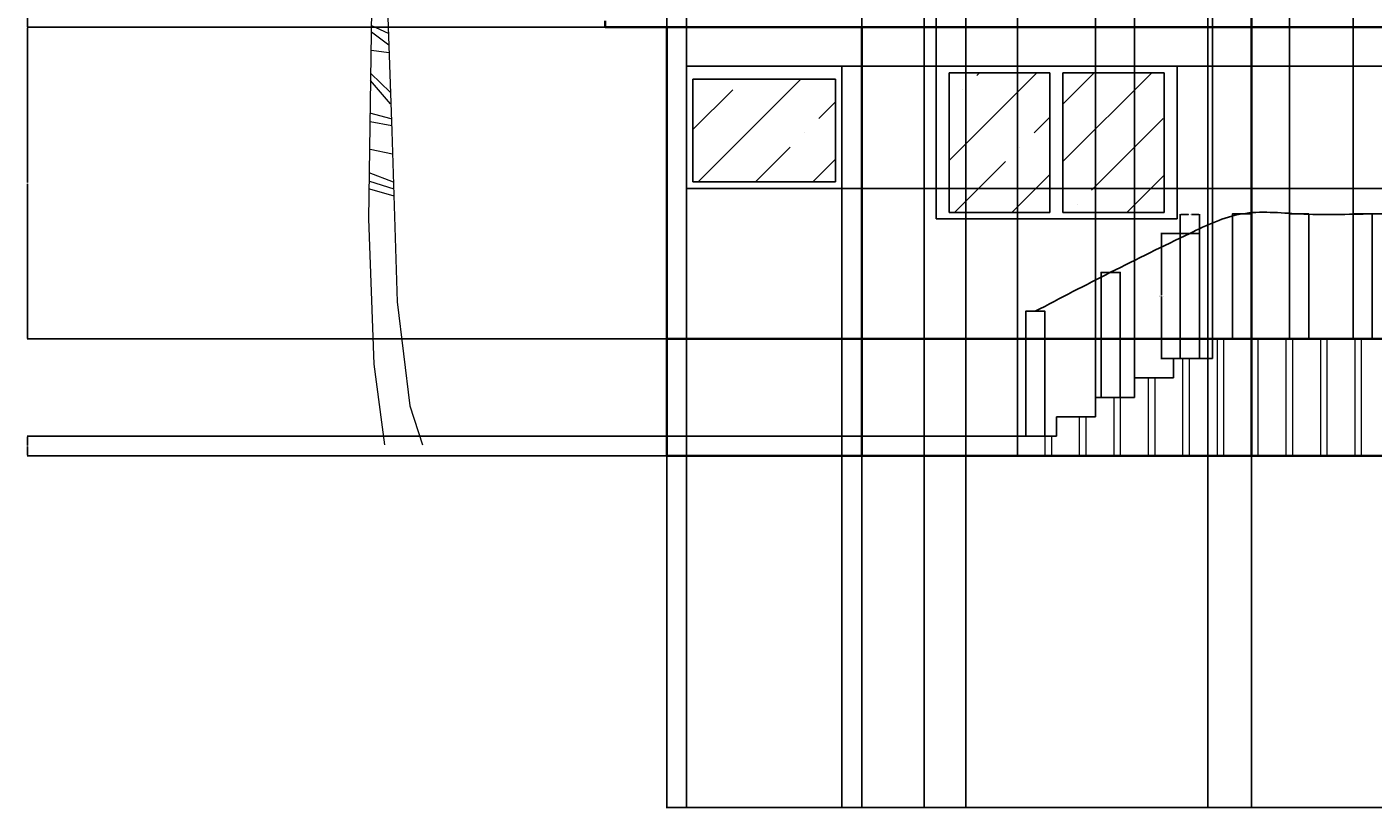
# Model space of a CAD drawing. Units: inches. Extents: x -177 to 697, y -125 to 346.
# Tile 1 of 4: x -177 to 237, y -125 to 116. Entities that reach past the tile are written whole.
import ezdxf

# ---------------------------------------------------------------- set-up
doc = ezdxf.new("R2010")
doc.units = ezdxf.units.IN
doc.header["$MEASUREMENT"] = 0
for name, color, linetype, lineweight in [('A-ANNO-DIMS', 2, 'Continuous', 18), ('A-FLOR-DECK', 8, 'Continuous', 18), ('A-FLOR-HRAL', 2, 'Continuous', 25), ('A-FLOR-STRS', 7, 'Continuous', 25), ('A-GLAZ', 4, 'Continuous', 25), ('A-GLAZ-PATT', 252, 'Continuous', 13), ('A-ROOF', 1, 'Continuous', 35), ('A-WALL', 7, 'Continuous', 35), ('L-PLNT', 94, 'Continuous', 13), ('S-FNDN', 7, 'Continuous', 35)]:
    doc.layers.add(name, color=color, linetype=linetype, lineweight=lineweight)
doc.styles.get("Standard").update_dxf_attribs({"font": 'arial.ttf'})
doc.dimstyles.get("Standard").update_dxf_attribs({"dimtxt": 0.18, "dimasz": 0.18, "dimexe": 0.18, "dimexo": 0.0625, "dimgap": 0.09, "dimtad": 0, "dimtih": 1, "dimtoh": 1, "dimdec": 4, "dimzin": 0, "dimdsep": 46, "dimtxsty": 'Standard', "dimcen": 0.09, "dimadec": 0, "dimazin": 0, "dimtfac": 1, "dimtdec": 4, "dimtofl": 0, "dimtmove": 0, "dimatfit": 3, "dimfxl": 1, "dimtolj": 1, "dimtzin": 0, "dimarcsym": 0})

# ---------------------------------------------------------------- blocks, each defined once
blk = doc.blocks.new('*U2')
for p, q in [((-7.5, 199.68), (-7.5, 197.946)), ((-5.567, 196.707), (-4.987, 201.167)), ((-4.407, 195.716), (-3.247, 200.672)), ((-2.474, 193.733), (-1.315, 199.433)), ((-6.727, 197.202), (-11.366, 197.45)), ((-3.441, 194.477), (-10.013, 195.716)), ((-1.121, 190.759), (0.232, 196.955)), ((9.317, 191.255), (10.283, 196.955)), ((11.829, 192.99), (13.182, 197.45)), ((13.956, 194.229), (14.729, 196.955)), ((15.116, 194.477), (17.822, 198.689)), ((16.082, 194.972), (17.822, 192.494)), ((18.015, 195.716), (20.914, 198.689)), ((18.015, 195.468), (18.981, 192.494)), ((19.368, 196.459), (19.948, 193.733)), ((20.914, 196.459), (21.301, 194.972)), ((21.301, 196.459), (22.847, 198.441)), ((22.074, 196.707), (23.427, 195.716)), ((23.234, 196.707), (23.62, 197.698)), ((-29.729, 190.759), (-31.469, 191.255)), ((-25.283, 191.751), (-29.342, 192.246)), ((-28.763, 190.759), (-28.763, 188.281)), ((-26.443, 191.503), (-26.636, 186.051)), ((-20.064, 191.751), (-25.863, 193.238)), ((-23.737, 191.751), (-24.51, 185.06)), ((-21.031, 191.998), (-21.804, 183.325)), ((-15.232, 191.255), (-20.644, 193.981)), ((-17.551, 191.503), (-20.451, 181.343)), ((-14.265, 190.759), (-18.131, 182.086)), ((-9.433, 189.025), (-15.618, 193.238)), ((-1.894, 192.494), (-9.24, 193.733)), ((-0.541, 189.52), (-7.307, 192.494)), ((0.038, 188.281), (1.778, 193.981)), ((1.005, 185.803), (2.358, 190.759)), ((5.837, 187.786), (7.577, 194.229)), ((11.25, 192.494), (15.889, 190.512)), ((14.536, 193.981), (17.242, 191.255)), ((-30.309, 190.512), (-30.695, 189.025)), ((-11.753, 189.768), (-15.425, 182.83)), ((-8.08, 188.034), (-12.912, 182.83)), ((-6.147, 186.299), (-9.24, 190.264)), ((-5.76, 190.016), (0.618, 185.308)), ((-5.76, 188.034), (-1.508, 182.582)), ((1.005, 182.582), (2.938, 186.547)), ((4.098, 185.06), (4.678, 190.512)), ((4.871, 186.051), (10.09, 186.547)), ((6.997, 188.529), (12.216, 187.786)), ((8.544, 190.512), (13.763, 189.52)), ((9.51, 184.317), (15.502, 188.034)), ((15.695, 186.299), (19.368, 188.777)), ((17.242, 186.547), (23.041, 180.599)), ((19.368, 187.29), (26.133, 189.768)), ((20.721, 187.042), (25.167, 181.343)), ((23.814, 187.29), (26.907, 181.343)), ((24.78, 187.538), (31.546, 188.777)), ((26.133, 187.29), (29.419, 181.838)), ((28.066, 187.29), (30.966, 182.582)), ((29.806, 186.795), (32.319, 183.078)), ((29.999, 186.795), (33.092, 187.29)), ((-4.987, 185.803), (-10.979, 182.086)), ((-3.247, 183.821), (-8.08, 181.838)), ((-2.668, 185.803), (1.198, 181.343)), ((2.938, 182.582), (6.61, 183.821)), ((4.871, 181.591), (8.544, 184.812)), ((7.77, 183.325), (16.082, 179.856)), ((11.25, 184.812), (17.628, 180.352)), ((14.536, 185.803), (19.948, 180.847)), ((32.512, 186.299), (35.218, 186.299)), ((33.479, 186.051), (34.445, 182.83)), ((35.605, 185.556), (37.151, 185.308)), ((35.798, 185.308), (36.958, 181.591)), ((38.118, 184.317), (38.504, 181.838)), ((39.857, 182.83), (40.244, 181.591)), ((-15.618, 179.36), (-20.644, 178.617)), ((-17.358, 178.617), (-13.299, 173.661)), ((-15.038, 179.36), (-10.786, 174.404)), ((-12.332, 180.104), (-9.433, 175.643)), ((-10.206, 180.104), (-8.08, 175.891)), ((-8.273, 180.104), (-6.147, 176.635)), ((-6.34, 179.608), (-4.6, 177.13)), ((-1.315, 181.591), (-5.374, 181.095)), ((-4.021, 179.36), (-2.861, 177.378)), ((-0.348, 180.352), (-1.894, 180.104)), ((4.098, 180.847), (8.35, 179.608)), ((5.644, 181.838), (13.569, 178.865)), ((7.384, 178.369), (10.476, 179.36)), ((11.829, 177.874), (18.015, 179.113)), ((18.015, 177.13), (26.133, 179.113)), ((-25.09, 175.148), (-28.376, 174.404)), ((-25.476, 174.652), (-21.224, 167.466)), ((-21.031, 177.626), (-24.897, 176.387)), ((-24.317, 175.891), (-18.711, 168.457)), ((-22.191, 176.635), (-16.391, 169.448)), ((-20.064, 177.626), (-15.812, 172.67)), ((-4.214, 175.148), (-14.072, 170.935)), ((-1.701, 176.882), (-8.66, 175.396)), ((-4.6, 174.9), (-4.021, 166.722)), ((-2.668, 176.387), (-2.376, 170.594)), ((-0.928, 176.882), (-1.508, 173.909)), ((2.551, 175.891), (-0.928, 171.431)), ((3.711, 174.404), (-0.541, 167.961)), ((1.585, 177.13), (0.038, 174.652)), ((1.585, 177.13), (6.61, 176.139)), ((2.938, 175.891), (8.737, 173.413)), ((6.224, 178.121), (8.157, 175.148)), ((8.157, 178.121), (10.476, 172.422)), ((10.476, 177.874), (12.796, 169.696)), ((13.182, 177.874), (14.729, 166.97)), ((15.889, 177.13), (16.855, 164.492)), ((18.981, 175.891), (19.561, 163.005)), ((20.914, 175.891), (30.966, 176.635)), ((21.688, 175.396), (22.074, 161.518)), ((23.814, 174.404), (25.554, 160.279)), ((-28.956, 172.174), (-32.435, 170.192)), ((-31.082, 169.944), (-32.435, 169.2)), ((-27.409, 173.413), (-30.695, 172.67)), ((-29.922, 170.687), (-27.989, 165.235)), ((-27.989, 172.422), (-26.056, 166.227)), ((-26.829, 173.661), (-23.544, 167.218)), ((-8.466, 171.678), (-16.585, 167.713)), ((-8.853, 170.935), (-7.113, 160.527)), ((-6.92, 172.917), (-5.374, 163.253)), ((5.257, 171.926), (-0.155, 163.005)), ((4.291, 173.909), (12.216, 168.953)), ((6.417, 170.439), (14.729, 164.492)), ((25.554, 173.661), (33.285, 173.661)), ((26.52, 173.165), (28.066, 159.784)), ((28.839, 172.174), (36.378, 170.687)), ((29.226, 171.926), (30.966, 158.545)), ((30.966, 170.687), (38.891, 167.713)), ((-32.628, 167.961), (-33.208, 167.961)), ((-32.628, 167.713), (-32.435, 165.979)), ((-31.662, 168.705), (-31.082, 165.483)), ((-12.139, 167.961), (-19.098, 162.014)), ((-12.719, 166.722), (-9.046, 154.828)), ((-10.979, 168.457), (-7.887, 157.801)), ((7.384, 168.705), (0.812, 157.553)), ((8.544, 165.979), (16.662, 160.527)), ((32.126, 169.696), (32.512, 158.545)), ((34.058, 168.705), (34.445, 158.545)), ((35.412, 167.713), (41.404, 164.988)), ((36.378, 166.474), (35.605, 158.792)), ((-14.265, 164.244), (-19.678, 158.049)), ((-14.265, 163.749), (-10.786, 154.828)), ((9.317, 164.244), (2.358, 154.332)), ((10.09, 162.51), (17.435, 157.058)), ((37.731, 165.235), (36.958, 159.288)), ((37.924, 165.235), (41.404, 163.749)), ((38.504, 164.492), (38.504, 159.536)), ((39.664, 163.253), (42.37, 161.766)), ((39.857, 162.757), (39.857, 160.031)), ((40.824, 161.766), (41.21, 160.031)), ((-16.005, 160.031), (-19.484, 154.084)), ((-16.585, 158.545), (-13.106, 152.35)), ((-15.618, 160.775), (-12.332, 154.332)), ((10.863, 159.784), (4.484, 152.35)), ((11.443, 157.553), (16.855, 154.332)), ((41.21, 161.518), (42.757, 160.279)), ((-18.131, 153.589), (-19.484, 151.606)), ((-17.358, 155.819), (-14.845, 151.358)), ((11.829, 155.075), (6.804, 150.119)), ((-17.938, 152.597), (-16.972, 151.111)), ((12.603, 151.111), (8.544, 148.385)), ((12.216, 153.093), (16.082, 151.606)), ((12.603, 149.872), (15.116, 149.128)), ((12.216, 148.137), (10.09, 147.393)), ((12.409, 145.659), (11.056, 145.659)), ((12.409, 146.898), (13.763, 146.402)), ((-4.081, 140.645), (0.753, 138.261)), ((-4.081, 137.547), (0.753, 135.163)), ((-4.081, 129.205), (1.124, 126.821)), ((-4.081, 127.298), (1.31, 123.246)), ((-4.081, 121.578), (1.31, 120.863)), ((-4.453, 112.283), (1.682, 105.133)), ((-4.267, 114.428), (1.682, 108.708)), ((-4.639, 102.273), (1.868, 100.604)), ((-4.453, 99.651), (2.24, 98.459)), ((-4.453, 91.071), (2.426, 89.641)), ((-4.825, 83.921), (2.612, 81.061)), ((-4.639, 81.299), (2.797, 78.916)), ((-4.639, 78.916), (2.797, 76.771))]:
    blk.add_line(p, q)
for points in [[(-2.363, 170.553), (-3.88, 148.505), (-4.988, 69.634), (-3.325, 24.869), (0, 0)], [(-0.116, 162.848), (0.554, 143.532), (2.217, 96.635), (3.88, 44.054), (7.76, 12.079), (11.64, 0)]]:
    blk.add_lwpolyline(points)
for centre, radius, start, end in [((-18.427, 181.448), 19.715, 350.285, 64.11229), ((25.595, 171.567), 25.395, 91.40319, 163.882), ((-21.738, 166.094), 25.899, 27.67115, 112.5305), ((23.687, 155.341), 32.188, 56.19272, 134.3213), ((-9.259, 151.732), 28.386, 68.38311, 147.5322), ((14.394, 148.393), 32.752, 113.7592, 177.4133), ((5.828, 132.718), 45.639, 35.98777, 95.82273), ((-32.8, 147.923), 45.309, 356.1943, 41.37848)]:
    blk.add_arc(centre, radius, start, end)
blk = doc.blocks.new('WIN-TWIN-LARGE-ELEV')
for p, q in [((0, 47.05), (74.16, 47.05)), ((0, 0), (0, 47.05)), ((74.16, 47.05), (74.16, 0)), ((4, 2), (4, 45.05)), ((4, 45.05), (35.01, 45.05)), ((35.01, 2), (35.01, 45.05)), ((39.01, 2), (39.01, 45.05)), ((39.01, 45.05), (70.16, 45.05)), ((70.16, 45.05), (70.16, 2)), ((74.16, 0), (0, 0)), ((35.01, 2), (4, 2)), ((70.16, 2), (39.01, 2))]:
    blk.add_line(p, q)
blk = doc.blocks.new('GUARD-POST-ELEV')
blk.add_lwpolyline([(5.89, 0), (0, 0), (0, 38.51), (5.89, 38.51)], close=True)
blk = doc.blocks.new('PORCH-UPRIGHT-36-ELEV')
for p, q in [((0, 36), (0, 0)), ((2, 36), (2, 0))]:
    blk.add_line(p, q)
blk = doc.blocks.new('*D15')
at = {"layer": 'A-ANNO-DIMS', "color": 0, "lineweight": -2, "transparency": 16777216}
for p, q in [((178.06, 52.19), (172.16, 52.19)), ((172.34, 52.01), (172.34, 33.12)), ((172.34, 13.86), (172.34, 32.75)), ((178.06, 13.68), (172.16, 13.68))]:
    blk.add_line(p, q, dxfattribs=at)
at = {"layer": 'A-ANNO-DIMS', "color": 0, "transparency": 16777216}
for points in [[(172.31, 52.01), (172.37, 52.01), (172.34, 52.19)], [(172.31, 13.86), (172.37, 13.86), (172.34, 13.68)]]:
    blk.add_solid(points, dxfattribs=at)
at = {"layer": 'Defpoints', "color": 0, "transparency": 16777216}
for p in [(172.34, 52.19), (178.12, 52.19), (178.12, 13.68)]:
    blk.add_point(p, dxfattribs=at)
at = {"layer": 'A-ANNO-DIMS', "color": 0, "transparency": 16777216, "insert": (172.34, 32.94), "char_height": 0.18, "attachment_point": 5}
blk.add_mtext('\\A1;POST 39 TYP.', dxfattribs=at)
blk = doc.blocks.new('*D16')
at = {"layer": 'A-ANNO-DIMS', "color": 0, "lineweight": -2, "transparency": 16777216}
for p, q in [((178.12, 52.26), (178.12, 58.15)), ((184.01, 52.26), (184.01, 58.15)), ((178.3, 57.97), (180.61, 57.97)), ((183.83, 57.97), (181.53, 57.97))]:
    blk.add_line(p, q, dxfattribs=at)
at = {"layer": 'A-ANNO-DIMS', "color": 0, "transparency": 16777216}
for points in [[(178.3, 58), (178.3, 57.94), (178.12, 57.97)], [(183.83, 58), (183.83, 57.94), (184.01, 57.97)]]:
    blk.add_solid(points, dxfattribs=at)
at = {"layer": 'Defpoints', "color": 0, "transparency": 16777216}
for p in [(184.01, 57.97), (178.12, 52.19), (184.01, 52.19)]:
    blk.add_point(p, dxfattribs=at)
at = {"layer": 'A-ANNO-DIMS', "color": 0, "transparency": 16777216, "insert": (181.07, 57.97), "char_height": 0.18, "attachment_point": 5}
blk.add_mtext('\\A1;6 TYP.', dxfattribs=at)
blk = doc.blocks.new('*D19')
at = {"layer": 'A-ANNO-DIMS', "color": 0, "lineweight": -2, "transparency": 16777216}
for p, q in [((20.05, -16.38), (20.05, -124.85)), ((500.05, -16.38), (500.05, -124.85)), ((20.23, -124.67), (259.76, -124.67)), ((499.87, -124.67), (260.34, -124.67))]:
    blk.add_line(p, q, dxfattribs=at)
at = {"layer": 'A-ANNO-DIMS', "color": 0, "transparency": 16777216}
for points in [[(20.23, -124.64), (20.23, -124.7), (20.05, -124.67)], [(499.87, -124.64), (499.87, -124.7), (500.05, -124.67)]]:
    blk.add_solid(points, dxfattribs=at)
at = {"layer": 'Defpoints', "color": 0, "transparency": 16777216}
for p in [(20.05, -16.32), (500.05, -16.32), (500.05, -124.67)]:
    blk.add_point(p, dxfattribs=at)
at = {"layer": 'A-ANNO-DIMS', "color": 0, "transparency": 16777216, "insert": (260.05, -124.67), "char_height": 0.18, "attachment_point": 5}
blk.add_mtext('\\A1;480', dxfattribs=at)
blk = doc.blocks.new('*D22')
at = {"layer": 'A-ANNO-DIMS', "color": 0, "lineweight": -2, "transparency": 16777216}
for p, q in [((79.79, 235.68), (-176.98, 235.68)), ((-176.8, 235.5), (-176.8, 175.86)), ((-176.8, 115.86), (-176.8, 175.5)), ((0.99, 115.68), (-176.98, 115.68))]:
    blk.add_line(p, q, dxfattribs=at)
at = {"layer": 'A-ANNO-DIMS', "color": 0, "transparency": 16777216}
for points in [[(-176.83, 235.5), (-176.77, 235.5), (-176.8, 235.68)], [(-176.83, 115.86), (-176.77, 115.86), (-176.8, 115.68)]]:
    blk.add_solid(points, dxfattribs=at)
at = {"layer": 'Defpoints', "color": 0, "transparency": 16777216}
for p in [(79.85, 235.68), (-176.8, 115.68), (1.05, 115.68)]:
    blk.add_point(p, dxfattribs=at)
at = {"layer": 'A-ANNO-DIMS', "color": 0, "transparency": 16777216, "insert": (-176.8, 175.68), "char_height": 0.18, "attachment_point": 5}
blk.add_mtext('\\A1;120', dxfattribs=at)
blk = doc.blocks.new('*D23')
at = {"layer": 'A-ANNO-DIMS', "color": 0, "lineweight": -2, "transparency": 16777216}
for p, q in [((19.99, 115.68), (-176.98, 115.68)), ((-176.8, 115.5), (-176.8, 67.86)), ((-176.8, 19.86), (-176.8, 67.5)), ((19.99, 19.68), (-176.98, 19.68))]:
    blk.add_line(p, q, dxfattribs=at)
at = {"layer": 'A-ANNO-DIMS', "color": 0, "transparency": 16777216}
for points in [[(-176.83, 115.5), (-176.77, 115.5), (-176.8, 115.68)], [(-176.83, 19.86), (-176.77, 19.86), (-176.8, 19.68)]]:
    blk.add_solid(points, dxfattribs=at)
at = {"layer": 'Defpoints', "color": 0, "transparency": 16777216}
for p in [(-176.8, 115.68), (20.05, 115.68), (20.05, 19.68)]:
    blk.add_point(p, dxfattribs=at)
at = {"layer": 'A-ANNO-DIMS', "color": 0, "transparency": 16777216, "insert": (-176.8, 67.68), "char_height": 0.18, "attachment_point": 5}
blk.add_mtext('\\A1;96', dxfattribs=at)
blk = doc.blocks.new('*D24')
at = {"layer": 'A-ANNO-DIMS', "color": 0, "lineweight": -2, "transparency": 16777216}
for p, q in [((128.05, -16.26), (128.05, 346.22)), ((128.23, 346.04), (157.83, 346.04)), ((187.87, 346.04), (158.27, 346.04)), ((188.05, 19.74), (188.05, 346.22))]:
    blk.add_line(p, q, dxfattribs=at)
at = {"layer": 'A-ANNO-DIMS', "color": 0, "transparency": 16777216}
for points in [[(128.23, 346.07), (128.23, 346.01), (128.05, 346.04)], [(187.87, 346.07), (187.87, 346.01), (188.05, 346.04)]]:
    blk.add_solid(points, dxfattribs=at)
at = {"layer": 'Defpoints', "color": 0, "transparency": 16777216}
for p in [(188.05, 346.04), (188.05, 19.68), (128.05, -16.32)]:
    blk.add_point(p, dxfattribs=at)
at = {"layer": 'A-ANNO-DIMS', "color": 0, "transparency": 16777216, "insert": (158.05, 346.04), "char_height": 0.18, "attachment_point": 5}
blk.add_mtext('\\A1;60', dxfattribs=at)
blk = doc.blocks.new('*D25')
at = {"layer": 'A-ANNO-DIMS', "color": 0, "lineweight": -2, "transparency": 16777216}
for p, q in [((152.05, 1.74), (152.05, 346.22)), ((152.23, 346.04), (157.84, 346.04)), ((163.87, 346.04), (158.26, 346.04)), ((164.05, 1.74), (164.05, 346.22))]:
    blk.add_line(p, q, dxfattribs=at)
at = {"layer": 'A-ANNO-DIMS', "color": 0, "transparency": 16777216}
for points in [[(152.23, 346.07), (152.23, 346.01), (152.05, 346.04)], [(163.87, 346.07), (163.87, 346.01), (164.05, 346.04)]]:
    blk.add_solid(points, dxfattribs=at)
at = {"layer": 'Defpoints', "color": 0, "transparency": 16777216}
for p in [(164.05, 346.04), (152.05, 1.68), (164.05, 1.68)]:
    blk.add_point(p, dxfattribs=at)
at = {"layer": 'A-ANNO-DIMS', "color": 0, "transparency": 16777216, "insert": (158.05, 346.04), "char_height": 0.18, "attachment_point": 5}
blk.add_mtext('\\A1;12', dxfattribs=at)
blk = doc.blocks.new('*D26')
at = {"layer": 'A-ANNO-DIMS', "color": 0, "lineweight": -2, "transparency": 16777216}
for p, q in [((127.99, -10.32), (-176.98, -10.32)), ((-176.8, -10.5), (-176.8, -13.14)), ((127.99, -16.32), (-176.98, -16.32)), ((-176.8, -16.14), (-176.8, -13.5))]:
    blk.add_line(p, q, dxfattribs=at)
at = {"layer": 'A-ANNO-DIMS', "color": 0, "transparency": 16777216}
for points in [[(-176.83, -10.5), (-176.77, -10.5), (-176.8, -10.32)], [(-176.83, -16.14), (-176.77, -16.14), (-176.8, -16.32)]]:
    blk.add_solid(points, dxfattribs=at)
at = {"layer": 'Defpoints', "color": 0, "transparency": 16777216}
for p in [(-176.8, -10.32), (128.05, -10.32), (128.05, -16.32)]:
    blk.add_point(p, dxfattribs=at)
at = {"layer": 'A-ANNO-DIMS', "color": 0, "transparency": 16777216, "insert": (-176.8, -13.32), "char_height": 0.18, "attachment_point": 5}
blk.add_mtext('\\A1;6', dxfattribs=at)
blk = doc.blocks.new('*D28')
at = {"layer": 'A-ANNO-DIMS', "color": 0, "lineweight": -2, "transparency": 16777216}
for p, q in [((211.79, 58.26), (211.79, 346.22)), ((211.97, 346.04), (221.1, 346.04)), ((231.15, 346.04), (222.01, 346.04)), ((231.33, 58.26), (231.33, 346.22))]:
    blk.add_line(p, q, dxfattribs=at)
at = {"layer": 'A-ANNO-DIMS', "color": 0, "transparency": 16777216}
for points in [[(211.97, 346.07), (211.97, 346.01), (211.79, 346.04)], [(231.15, 346.07), (231.15, 346.01), (231.33, 346.04)]]:
    blk.add_solid(points, dxfattribs=at)
at = {"layer": 'Defpoints', "color": 0, "transparency": 16777216}
for p in [(231.33, 346.04), (211.79, 58.19), (231.33, 58.19)]:
    blk.add_point(p, dxfattribs=at)
at = {"layer": 'A-ANNO-DIMS', "color": 0, "transparency": 16777216, "insert": (221.56, 346.04), "char_height": 0.18, "attachment_point": 5}
blk.add_mtext('\\A1;19.536', dxfattribs=at)
blk = doc.blocks.new('*D30')
at = {"layer": 'A-ANNO-DIMS', "color": 0, "lineweight": -2, "transparency": 16777216}
for p, q in [((20.05, 115.62), (20.05, -124.85)), ((80.05, 115.62), (80.05, -124.85)), ((20.23, -124.67), (49.83, -124.67)), ((79.87, -124.67), (50.27, -124.67))]:
    blk.add_line(p, q, dxfattribs=at)
at = {"layer": 'A-ANNO-DIMS', "color": 0, "transparency": 16777216}
for points in [[(20.23, -124.64), (20.23, -124.7), (20.05, -124.67)], [(79.87, -124.64), (79.87, -124.7), (80.05, -124.67)]]:
    blk.add_solid(points, dxfattribs=at)
at = {"layer": 'Defpoints', "color": 0, "transparency": 16777216}
for p in [(20.05, 115.68), (80.05, 115.68), (80.05, -124.67)]:
    blk.add_point(p, dxfattribs=at)
at = {"layer": 'A-ANNO-DIMS', "color": 0, "transparency": 16777216, "insert": (50.05, -124.67), "char_height": 0.18, "attachment_point": 5}
blk.add_mtext('\\A1;60', dxfattribs=at)
blk = doc.blocks.new('*D31')
at = {"layer": 'A-ANNO-DIMS', "color": 0, "lineweight": -2, "transparency": 16777216}
for p, q in [((80.05, -16.26), (80.05, 346.22)), ((80.23, 346.04), (103.83, 346.04)), ((127.87, 346.04), (104.27, 346.04)), ((128.05, -16.26), (128.05, 346.22))]:
    blk.add_line(p, q, dxfattribs=at)
at = {"layer": 'A-ANNO-DIMS', "color": 0, "transparency": 16777216}
for points in [[(80.23, 346.07), (80.23, 346.01), (80.05, 346.04)], [(127.87, 346.07), (127.87, 346.01), (128.05, 346.04)]]:
    blk.add_solid(points, dxfattribs=at)
at = {"layer": 'Defpoints', "color": 0, "transparency": 16777216}
for p in [(128.05, 346.04), (80.05, -16.32), (128.05, -16.32)]:
    blk.add_point(p, dxfattribs=at)
at = {"layer": 'A-ANNO-DIMS', "color": 0, "transparency": 16777216, "insert": (104.05, 346.04), "char_height": 0.18, "attachment_point": 5}
blk.add_mtext('\\A1;48', dxfattribs=at)
blk = doc.blocks.new('*D36')
at = {"layer": 'A-ANNO-DIMS', "color": 0, "lineweight": -2, "transparency": 16777216}
for p, q in [((26.06, 66), (26.06, -124.85)), ((73.94, 66), (73.94, -124.85)), ((26.24, -124.67), (49.6, -124.67)), ((73.76, -124.67), (50.4, -124.67))]:
    blk.add_line(p, q, dxfattribs=at)
at = {"layer": 'A-ANNO-DIMS', "color": 0, "transparency": 16777216}
for points in [[(26.24, -124.64), (26.24, -124.7), (26.06, -124.67)], [(73.76, -124.64), (73.76, -124.7), (73.94, -124.67)]]:
    blk.add_solid(points, dxfattribs=at)
at = {"layer": 'Defpoints', "color": 0, "transparency": 16777216}
for p in [(26.06, 66.06), (73.94, 66.06), (73.94, -124.67)]:
    blk.add_point(p, dxfattribs=at)
at = {"layer": 'A-ANNO-DIMS', "color": 0, "transparency": 16777216, "insert": (50, -124.67), "char_height": 0.18, "attachment_point": 5}
blk.add_mtext('\\A1;47.88', dxfattribs=at)
blk = doc.blocks.new('*D37')
at = {"layer": 'A-ANNO-DIMS', "color": 0, "lineweight": -2, "transparency": 16777216}
for p, q in [((74.01, 103.68), (697.14, 103.68)), ((696.96, 103.5), (696.96, 85.05)), ((696.96, 66.24), (696.96, 84.69)), ((74.01, 66.06), (697.14, 66.06))]:
    blk.add_line(p, q, dxfattribs=at)
at = {"layer": 'A-ANNO-DIMS', "color": 0, "transparency": 16777216}
for points in [[(696.93, 103.5), (696.99, 103.5), (696.96, 103.68)], [(696.93, 66.24), (696.99, 66.24), (696.96, 66.06)]]:
    blk.add_solid(points, dxfattribs=at)
at = {"layer": 'Defpoints', "color": 0, "transparency": 16777216}
for p in [(73.94, 103.68), (696.96, 103.68), (73.94, 66.06)]:
    blk.add_point(p, dxfattribs=at)
at = {"layer": 'A-ANNO-DIMS', "color": 0, "transparency": 16777216, "insert": (696.96, 84.87), "char_height": 0.18, "attachment_point": 5}
blk.add_mtext('\\A1;37.62', dxfattribs=at)
blk = doc.blocks.new('*D38')
at = {"layer": 'A-ANNO-DIMS', "color": 0, "lineweight": -2, "transparency": 16777216}
for p, q in [((20.05, 19.74), (20.05, 346.22)), ((20.23, 346.04), (22.75, 346.04)), ((25.88, 346.04), (23.36, 346.04)), ((26.06, 66.12), (26.06, 346.22))]:
    blk.add_line(p, q, dxfattribs=at)
at = {"layer": 'A-ANNO-DIMS', "color": 0, "transparency": 16777216}
for points in [[(20.23, 346.07), (20.23, 346.01), (20.05, 346.04)], [(25.88, 346.07), (25.88, 346.01), (26.06, 346.04)]]:
    blk.add_solid(points, dxfattribs=at)
at = {"layer": 'Defpoints', "color": 0, "transparency": 16777216}
for p in [(26.06, 346.04), (26.06, 66.06), (20.05, 19.68)]:
    blk.add_point(p, dxfattribs=at)
at = {"layer": 'A-ANNO-DIMS', "color": 0, "transparency": 16777216, "insert": (23.05, 346.04), "char_height": 0.18, "attachment_point": 5}
blk.add_mtext('\\A1;6.01', dxfattribs=at)
blk = doc.blocks.new('*D39')
at = {"layer": 'A-ANNO-DIMS', "color": 0, "lineweight": -2, "transparency": 16777216}
for p, q in [((80.05, -16.26), (80.05, 346.22)), ((80.23, 346.04), (91.11, 346.04)), ((102.79, 346.04), (91.9, 346.04)), ((102.97, 56.7), (102.97, 346.22))]:
    blk.add_line(p, q, dxfattribs=at)
at = {"layer": 'A-ANNO-DIMS', "color": 0, "transparency": 16777216}
for points in [[(80.23, 346.07), (80.23, 346.01), (80.05, 346.04)], [(102.79, 346.07), (102.79, 346.01), (102.97, 346.04)]]:
    blk.add_solid(points, dxfattribs=at)
at = {"layer": 'Defpoints', "color": 0, "transparency": 16777216}
for p in [(102.97, 346.04), (102.97, 56.63), (80.05, -16.32)]:
    blk.add_point(p, dxfattribs=at)
at = {"layer": 'A-ANNO-DIMS', "color": 0, "transparency": 16777216, "insert": (91.51, 346.04), "char_height": 0.18, "attachment_point": 5}
blk.add_mtext('\\A1;22.92', dxfattribs=at)
blk = doc.blocks.new('*D46')
at = {"layer": 'A-ANNO-DIMS', "color": 0, "lineweight": -2, "transparency": 16777216}
for p, q in [((112.1, 190.16), (112.1, -124.85)), ((186.62, 190.16), (186.62, -124.85)), ((112.28, -124.67), (148.96, -124.67)), ((186.44, -124.67), (149.75, -124.67))]:
    blk.add_line(p, q, dxfattribs=at)
at = {"layer": 'A-ANNO-DIMS', "color": 0, "transparency": 16777216}
for points in [[(112.28, -124.64), (112.28, -124.7), (112.1, -124.67)], [(186.44, -124.64), (186.44, -124.7), (186.62, -124.67)]]:
    blk.add_solid(points, dxfattribs=at)
at = {"layer": 'Defpoints', "color": 0, "transparency": 16777216}
for p in [(112.1, 190.22), (186.62, 190.22), (186.62, -124.67)]:
    blk.add_point(p, dxfattribs=at)
at = {"layer": 'A-ANNO-DIMS', "color": 0, "transparency": 16777216, "insert": (149.36, -124.67), "char_height": 0.18, "attachment_point": 5}
blk.add_mtext('\\A1;74.52', dxfattribs=at)
blk = doc.blocks.new('*D51')
at = {"layer": 'A-ANNO-DIMS', "color": 0, "lineweight": -2, "transparency": 16777216}
for p, q in [((99.22, 235.62), (99.22, -124.85)), ((200.05, 235.62), (200.05, -124.85)), ((99.4, -124.67), (149.18, -124.67)), ((199.87, -124.67), (150.09, -124.67))]:
    blk.add_line(p, q, dxfattribs=at)
at = {"layer": 'A-ANNO-DIMS', "color": 0, "transparency": 16777216}
for points in [[(99.4, -124.64), (99.4, -124.7), (99.22, -124.67)], [(199.87, -124.64), (199.87, -124.7), (200.05, -124.67)]]:
    blk.add_solid(points, dxfattribs=at)
at = {"layer": 'Defpoints', "color": 0, "transparency": 16777216}
for p in [(99.22, 235.68), (200.05, 235.68), (200.05, -124.67)]:
    blk.add_point(p, dxfattribs=at)
at = {"layer": 'A-ANNO-DIMS', "color": 0, "transparency": 16777216, "insert": (149.63, -124.67), "char_height": 0.18, "attachment_point": 5}
blk.add_mtext('\\A1;100.83', dxfattribs=at)
blk = doc.blocks.new('*D55')
at = {"layer": 'A-ANNO-DIMS', "color": 0, "lineweight": -2, "transparency": 16777216}
for p, q in [((20.05, 115.74), (20.05, 346.22)), ((20.23, 346.04), (59.24, 346.04)), ((99.04, 346.04), (60.03, 346.04)), ((99.22, 163.74), (99.22, 346.22))]:
    blk.add_line(p, q, dxfattribs=at)
at = {"layer": 'A-ANNO-DIMS', "color": 0, "transparency": 16777216}
for points in [[(20.23, 346.07), (20.23, 346.01), (20.05, 346.04)], [(99.04, 346.07), (99.04, 346.01), (99.22, 346.04)]]:
    blk.add_solid(points, dxfattribs=at)
at = {"layer": 'Defpoints', "color": 0, "transparency": 16777216}
for p in [(99.22, 346.04), (99.22, 163.68), (20.05, 115.68)]:
    blk.add_point(p, dxfattribs=at)
at = {"layer": 'A-ANNO-DIMS', "color": 0, "transparency": 16777216, "insert": (59.63, 346.04), "char_height": 0.18, "attachment_point": 5}
blk.add_mtext('\\A1;79.17', dxfattribs=at)

msp = doc.modelspace()

# ---------------------------------------------------------------- hatches: boundary and pattern name
at = {"layer": 'A-GLAZ-PATT'}
h = msp.add_hatch(dxfattribs=at)
h.set_pattern_fill('ANSI35', color=256, scale=100)
h.set_pattern_definition([(45, (-118.808, -115.734), (-17.6777, 17.6777), []), (45, (-101.13, -115.734), (-17.6777, 17.6777), [31.25, -6.25, 0, -6.25])])
h.paths.add_polyline_path([(71.9429, 99.6802), (28.0592, 99.6802), (28.0592, 68.059), (71.9429, 68.059)])
h.paths.add_polyline_path([(137.9807, 101.6802), (106.9675, 101.6802), (106.9675, 58.6343), (137.9807, 58.6343)])
h.paths.add_polyline_path([(173.1317, 101.6802), (141.9807, 101.6802), (141.9807, 58.6343), (173.1317, 58.6343)])

# ---------------------------------------------------------------- linework, layer by layer
at = {"layer": 'A-FLOR-DECK'}
for p, q in [((178.8407, 13.6802), (178.8407, -16.3198)), ((180.8407, 13.6802), (180.8407, -16.3198)), ((168.2363, 7.6802), (168.2363, -16.3198)), ((170.2363, 7.6802), (170.2363, -16.3198)), ((157.6319, 1.6802), (157.6319, -16.3198)), ((159.6319, 1.6802), (159.6319, -16.3198)), ((147.0275, -4.3198), (147.0275, -16.3198)), ((147.0275, -4.3198), (147.0275, -16.3198)), ((149.0275, -4.3198), (149.0275, -16.3198)), ((149.0275, -4.3198), (149.0275, -16.3198)), ((136.423, -10.3198), (136.423, -16.3198)), ((138.423, -10.3198), (138.423, -16.3198))]:
    msp.add_line(p, q, dxfattribs=at)
at = {"layer": 'A-FLOR-HRAL'}
msp.add_open_spline([(133.4757, 28.1928), (141.2082, 32.2346), (156.9836, 40.4804), (177.8872, 50.6849), (196.9965, 59.8479), (216.4528, 57.5999), (235.2353, 58.3169), (254.7984, 58.158), (273.345, 58.2027), (293.4178, 58.1899), (312.9537, 58.1935), (332.4903, 58.1926), (351.4925, 58.1928), (364.5168, 58.1928), (371.029, 58.1928)], degree=3, knots=[0, 0, 0, 0, 26.12758735, 53.30341094, 70.42401933, 88.05900671, 110.54286492, 127.13195594, 146.66843056, 166.20490518, 187.34399835, 205.27785442, 224.81432904, 244.35080366, 244.35080366, 244.35080366, 244.35080366], dxfattribs=at)
at = {"layer": 'A-FLOR-STRS'}
for p, q in [((200.0496, 19.6802), (188.0496, 19.6802)), ((188.0496, 19.6802), (188.0496, 13.6802)), ((188.0496, 13.6802), (176.0496, 13.6802)), ((176.0496, 13.6802), (176.0496, 7.6802)), ((176.0496, 7.6802), (164.0496, 7.6802)), ((164.0496, 7.6802), (164.0496, 1.6802)), ((164.0496, 1.6802), (152.0496, 1.6802)), ((152.0496, 1.6802), (152.0496, -4.3198)), ((152.0496, -4.3198), (140.0496, -4.3198)), ((140.0496, -4.3198), (140.0496, -10.3198)), ((140.0496, -10.3198), (128.0496, -10.3198)), ((128.0496, -10.3198), (128.0496, -16.3198)), ((128.0496, -16.3198), (116.0496, -16.3198))]:
    msp.add_line(p, q, dxfattribs=at)
at = {"layer": 'A-GLAZ'}
for p, q in [((26.0592, 103.6802), (73.9429, 103.6802)), ((26.0592, 66.059), (26.0592, 103.6802)), ((73.9429, 103.6802), (73.9429, 66.059)), ((28.0592, 99.6802), (71.9429, 99.6802)), ((28.0592, 68.059), (28.0592, 99.6802)), ((71.9429, 99.6802), (71.9429, 68.059)), ((71.9429, 68.059), (28.0592, 68.059)), ((73.9429, 66.059), (26.0592, 66.059))]:
    msp.add_line(p, q, dxfattribs=at)
at = {"layer": 'A-ROOF'}
for p, q in [((1.0496, 117.6802), (1.0496, 115.6802)), ((1.0496, 115.6802), (20.0496, 115.6802)), ((20.0496, 115.6802), (500.0496, 115.6802))]:
    msp.add_line(p, q, dxfattribs=at)
at = {"layer": 'A-WALL'}
for p, q in [((200.0496, -16.3198), (200.0496, 235.6802)), ((20.0496, -16.3198), (20.0496, 115.6802)), ((80.0496, -16.3198), (80.0496, 115.6802))]:
    msp.add_line(p, q, dxfattribs=at)
at = {"layer": 'S-FNDN'}
for p, q in [((20.0496, 19.6802), (500.0496, 19.6802)), ((500.0496, -16.3198), (20.0496, -16.3198))]:
    msp.add_line(p, q, dxfattribs=at)

# ---------------------------------------------------------------- block references
at = {"layer": 'A-FLOR-DECK'}
for p in [(189.4452, -16.3198), (200.0496, -16.3198), (200.0496, -16.3198), (210.654, -16.3198), (221.2584, -16.3198), (231.8629, -16.3198)]:
    msp.add_blockref('PORCH-UPRIGHT-36-ELEV', p, dxfattribs=at)
at = {"layer": 'A-FLOR-HRAL'}
for p in [(194.1548, 19.6802), (211.7898, 19.6802), (231.3263, 19.6802), (178.12, 13.6802), (153.7371, 1.6802), (130.5283, -10.3198)]:
    msp.add_blockref('GUARD-POST-ELEV', p, dxfattribs=at)
at = {"layer": 'A-GLAZ'}
msp.add_blockref('WIN-TWIN-LARGE-ELEV', (102.9675, 56.6343), dxfattribs=at)
at = {"layer": 'L-PLNT'}
msp.add_blockref('*U2', (-66.8579, -12.984), dxfattribs=at)

# ---------------------------------------------------------------- dimensions: what is measured, and where the dimension line sits
at = {"layer": 'A-ANNO-DIMS'}
for base, p1, p2, override, picture, middle in [((26.0592, 346.0391), (20.0496, 19.6802), (26.0592, 66.059), {"dimdec": 2, "dimlfac": 1, "dimrnd": 0, "dimzin": 0, "dimdsep": 46, "dimlunit": 2}, '*D38', (23.0544, 346.0391)), ((99.2186, 346.0391), (20.0496, 115.6802), (99.2186, 163.6802), {"dimdec": 2, "dimlfac": 1, "dimrnd": 0, "dimzin": 0, "dimdsep": 46, "dimlunit": 2}, '*D55', (59.6341, 346.0391)), ((128.0496, 346.0391), (80.0496, -16.3198), (128.0496, -16.3198), {"dimdec": 0, "dimlfac": 1, "dimrnd": 0, "dimzin": 0, "dimdsep": 46, "dimlunit": 2}, '*D31', (104.0496, 346.0391)), ((102.9675, 346.0391), (80.0496, -16.3198), (102.9675, 56.6343), {"dimdec": 2, "dimlfac": 1, "dimrnd": 0, "dimzin": 0, "dimdsep": 46, "dimlunit": 2}, '*D39', (91.5085, 346.0391)), ((188.0496, 346.0391), (128.0496, -16.3198), (188.0496, 19.6802), {"dimdec": 0, "dimlfac": 1, "dimrnd": 0, "dimzin": 0, "dimdsep": 46, "dimlunit": 2}, '*D24', (158.0496, 346.0391)), ((164.0496, 346.0391), (152.0496, 1.6802), (164.0496, 1.6802), {"dimdec": 0, "dimlfac": 1, "dimrnd": 0, "dimzin": 0, "dimdsep": 46, "dimlunit": 2}, '*D25', (158.0496, 346.0391)), ((231.32629, 346.03909), (211.78981, 58.1928), (231.32629, 58.1928), {"dimdec": 3, "dimlfac": 1, "dimrnd": 0, "dimzin": 0, "dimdsep": 46, "dimlunit": 2}, '*D28', (221.55805, 346.03909)), ((200.0496, -124.671), (99.2186, 235.6802), (200.0496, 235.6802), {"dimdec": 2, "dimlfac": 1, "dimrnd": 0, "dimzin": 0, "dimdsep": 46, "dimlunit": 2}, '*D51', (149.6341, -124.671)), ((186.617, -124.671), (112.0968, 190.2226), (186.617, 190.2226), {"dimdec": 2, "dimlfac": 1, "dimrnd": 0, "dimzin": 0, "dimdsep": 46, "dimlunit": 2}, '*D46', (149.3569, -124.671)), ((80.0496, -124.671), (20.0496, 115.6802), (80.0496, 115.6802), {"dimdec": 0, "dimlfac": 1, "dimrnd": 0, "dimzin": 0, "dimdsep": 46, "dimlunit": 2}, '*D30', (50.0496, -124.671)), ((73.9429, -124.671), (26.0592, 66.059), (73.9429, 66.059), {"dimdec": 2, "dimlfac": 1, "dimrnd": 0, "dimzin": 0, "dimdsep": 46, "dimlunit": 2}, '*D36', (50.0011, -124.671)), ((500.0496, -124.671), (20.0496, -16.3198), (500.0496, -16.3198), {"dimdec": 0, "dimlfac": 1, "dimrnd": 0, "dimzin": 0, "dimdsep": 46, "dimlunit": 2}, '*D19', (260.0496, -124.671))]:
    dim = msp.add_linear_dim(base=base, p1=p1, p2=p2, dimstyle='Standard', override=override, dxfattribs=at)
    dim.commit()
    dim.dimension.update_dxf_attribs({"geometry": picture, "text_midpoint": middle})
for base, p1, p2, override, picture, middle in [((-176.8039, 115.6802), (79.8545, 235.6802), (1.0496, 115.6802), {"dimdec": 0, "dimlfac": 1, "dimrnd": 0, "dimzin": 0, "dimdsep": 46, "dimlunit": 2}, '*D22', (-176.8039, 175.6802)), ((-176.8039, 115.6802), (20.0496, 19.6802), (20.0496, 115.6802), {"dimdec": 0, "dimlfac": 1, "dimrnd": 0, "dimzin": 0, "dimdsep": 46, "dimlunit": 2}, '*D23', (-176.8039, 67.6802)), ((696.9617, 103.6802), (73.9429, 66.059), (73.9429, 103.6802), {"dimdec": 2, "dimlfac": 1, "dimrnd": 0, "dimzin": 0, "dimdsep": 46, "dimlunit": 2}, '*D37', (696.9617, 84.8696)), ((-176.8039, -10.3198), (128.0496, -16.3198), (128.0496, -10.3198), {"dimdec": 0, "dimlfac": 1, "dimrnd": 0, "dimzin": 0, "dimdsep": 46, "dimlunit": 2}, '*D26', (-176.8039, -13.3198))]:
    dim = msp.add_linear_dim(base=base, p1=p1, p2=p2, angle=90, dimstyle='Standard', override=override, dxfattribs=at)
    dim.commit()
    dim.dimension.update_dxf_attribs({"geometry": picture, "text_midpoint": middle})
dim = msp.add_linear_dim(base=(184.0148, 57.9697), p1=(178.12, 52.1928), p2=(184.0148, 52.1928), text='<> TYP.', dimstyle='Standard', override={"dimdec": 0, "dimlfac": 1, "dimrnd": 0, "dimzin": 0, "dimdsep": 46, "dimlunit": 2}, dxfattribs=at)
dim.commit()
dim.dimension.update_dxf_attribs({"geometry": '*D16', "text_midpoint": (181.0674, 57.9697)})
dim = msp.add_linear_dim(base=(172.3431, 52.1928), p1=(178.12, 13.6802), p2=(178.12, 52.1928), angle=90, text='POST <> TYP.', dimstyle='Standard', override={"dimdec": 0, "dimlfac": 1, "dimrnd": 0, "dimzin": 0, "dimdsep": 46, "dimlunit": 2}, dxfattribs=at)
dim.commit()
dim.dimension.update_dxf_attribs({"geometry": '*D15', "text_midpoint": (172.3431, 32.9365)})

doc.saveas('drawing.dxf')
